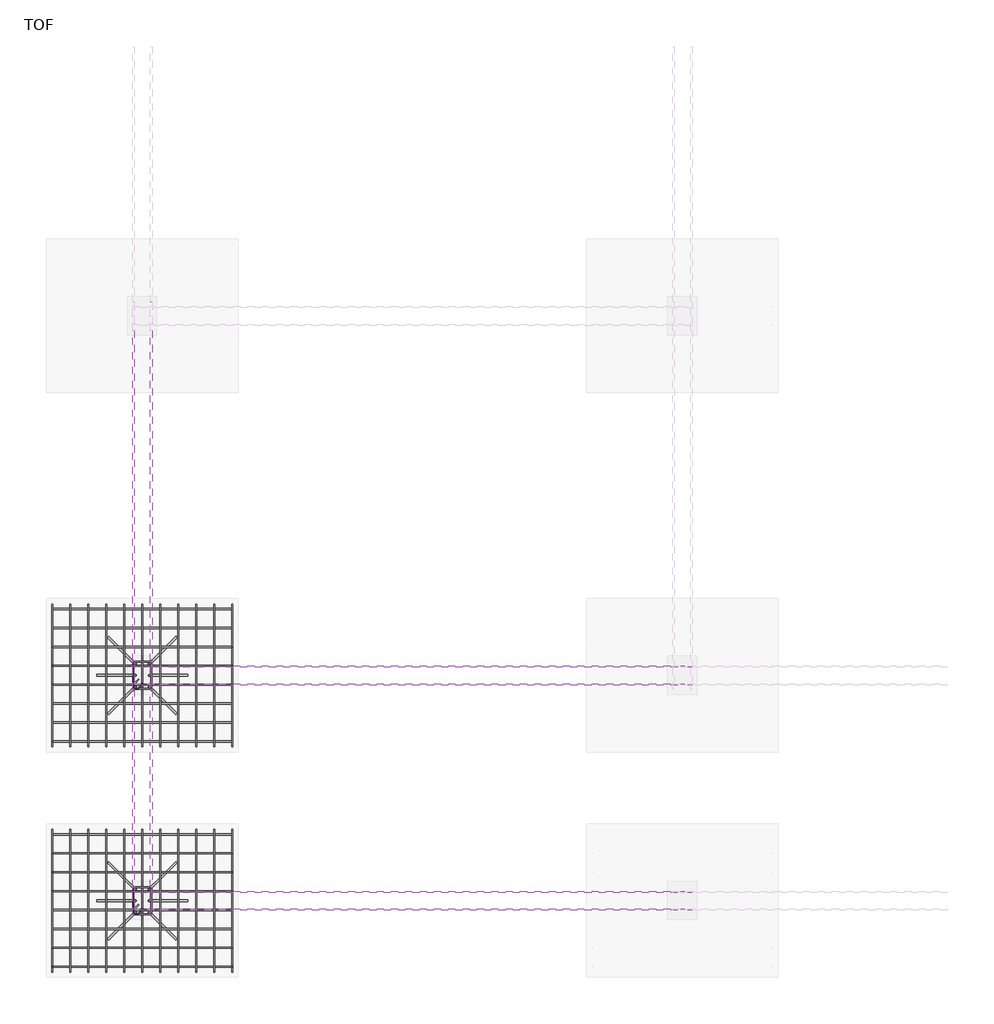
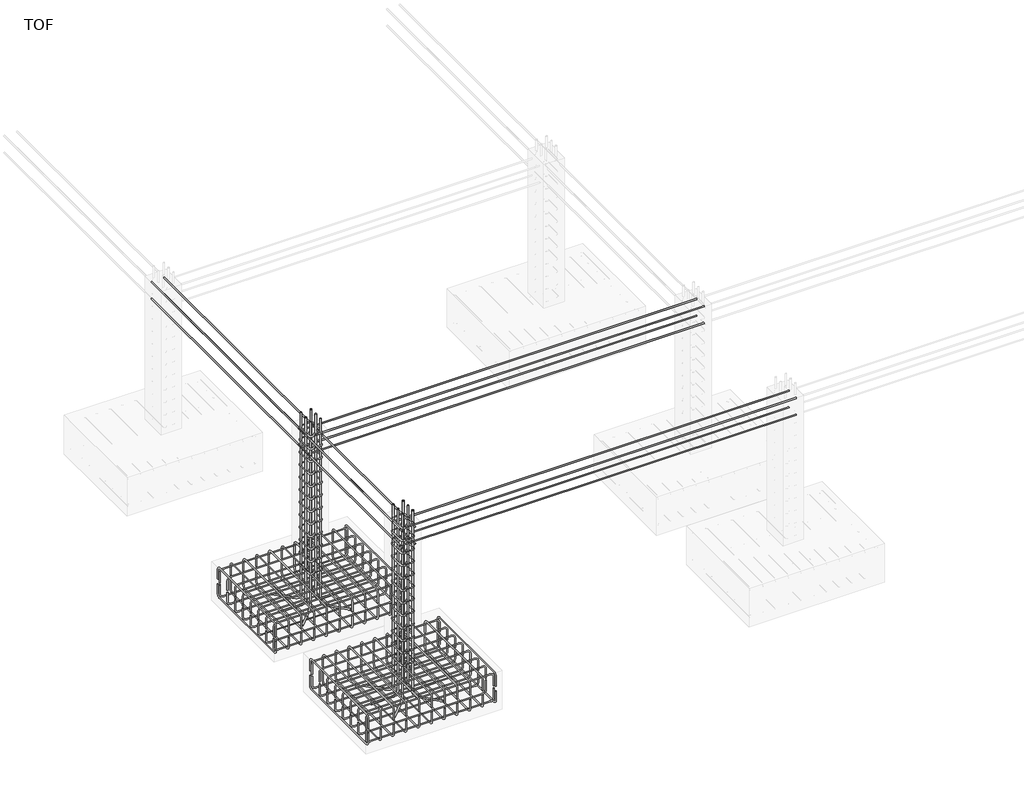
# One storey, part 2 of 10: 38 reinforcing bars.
"""IFC4 building model written with IfcOpenShell, lengths in millimetres."""

from ifc_helpers import new_model, si_unit, point, frame, origin, place, context, project, spatial, polyline, circle_curve, trimmed, segment, composite_curve, source, transform, mapped, element, save
from ifc_brep_helpers import swept_disk

model = new_model("IFC4")

# Units and contexts
model_context = context("Model", 3, world=origin())
ifc_project = project(units=[si_unit("LENGTHUNIT", "METRE", prefix="MILLI")], contexts=[model_context])

# Site, building, storey
site = spatial("IfcSite", under=ifc_project)
building = spatial("IfcBuilding", under=site)
storey = spatial("IfcBuildingStorey", under=building, Name="TOF", Elevation=-1828.8)

# Reinforcing bars
placement = place(None, origin())
reinforcing_bar_shape = source(origin(), model_context, "Body", "SolidModel", [
    swept_disk(composite_curve([segment(polyline([(-1914.7217857, -14539.6267376, -2018.8), (-1914.7217857, -14539.6267376, -1908.8)]), True, "CONTINUOUS"), segment(trimmed(circle_curve(frame((-1914.7217857, -14574.6267376, -1908.8), z_axis=(1.0, 0.0, 0.0), x_axis=(0.0, 35.0, 0.0)), 35.0), [point((-1914.7217857, -14539.6267376, -1908.8))], [point((-1914.7217857, -14574.6267376, -1873.8))], True, "CARTESIAN"), True, "CONTINUOUS"), segment(polyline([(-1914.7217857, -14574.6267376, -1873.8), (-1914.7217857, -15614.6267376, -1873.8)]), True, "CONTINUOUS"), segment(trimmed(circle_curve(frame((-1914.7217857, -15614.6267376, -1908.8), z_axis=(1.0, 0.0, 0.0), x_axis=(0.0, 0.0, 35.0)), 35.0), [point((-1914.7217857, -15614.6267376, -1873.8))], [point((-1914.7217857, -15649.6267376, -1908.8))], True, "CARTESIAN"), True, "CONTINUOUS"), segment(polyline([(-1914.7217857, -15649.6267376, -1908.8), (-1914.7217857, -15649.6267376, -2018.8)]), True, "CONTINUOUS")], self_intersect=False), 5.0),
])
element("IfcReinforcingBar", 1, at=placement, inside=storey, context=model_context, shape_type="MappedRepresentation", body=[
    mapped(reinforcing_bar_shape, transform((0.0, 0.0, 0.0), x_axis=(1.0, 0.0, 0.0), y_axis=(0.0, 1.0, 0.0), z_axis=(0.0, 0.0, 1.0))),
    mapped(reinforcing_bar_shape, transform((-141.0, 0.0, 0.0), x_axis=(1.0, 0.0, 0.0), y_axis=(0.0, 1.0, 0.0), z_axis=(0.0, 0.0, 1.0))),
    mapped(reinforcing_bar_shape, transform((-282.0, 0.0, 0.0), x_axis=(1.0, 0.0, 0.0), y_axis=(0.0, 1.0, 0.0), z_axis=(0.0, 0.0, 1.0))),
    mapped(reinforcing_bar_shape, transform((-423.0, 0.0, 0.0), x_axis=(1.0, 0.0, 0.0), y_axis=(0.0, 1.0, 0.0), z_axis=(0.0, 0.0, 1.0))),
    mapped(reinforcing_bar_shape, transform((-564.0, 0.0, 0.0), x_axis=(1.0, 0.0, 0.0), y_axis=(0.0, 1.0, 0.0), z_axis=(0.0, 0.0, 1.0))),
    mapped(reinforcing_bar_shape, transform((-705.0, 0.0, 0.0), x_axis=(1.0, 0.0, 0.0), y_axis=(0.0, 1.0, 0.0), z_axis=(0.0, 0.0, 1.0))),
    mapped(reinforcing_bar_shape, transform((-846.0, 0.0, 0.0), x_axis=(1.0, 0.0, 0.0), y_axis=(0.0, 1.0, 0.0), z_axis=(0.0, 0.0, 1.0))),
    mapped(reinforcing_bar_shape, transform((-987.0, 0.0, 0.0), x_axis=(1.0, 0.0, 0.0), y_axis=(0.0, 1.0, 0.0), z_axis=(0.0, 0.0, 1.0))),
    mapped(reinforcing_bar_shape, transform((-1128.0, 0.0, 0.0), x_axis=(1.0, 0.0, 0.0), y_axis=(0.0, 1.0, 0.0), z_axis=(0.0, 0.0, 1.0))),
    mapped(reinforcing_bar_shape, transform((-1269.0, 0.0, 0.0), x_axis=(1.0, 0.0, 0.0), y_axis=(0.0, 1.0, 0.0), z_axis=(0.0, 0.0, 1.0))),
    mapped(reinforcing_bar_shape, transform((-1410.0, 0.0, 0.0), x_axis=(1.0, 0.0, 0.0), y_axis=(0.0, 1.0, 0.0), z_axis=(0.0, 0.0, 1.0))),
])
reinforcing_bar_2_shape = source(origin(), model_context, "Body", "SolidModel", [
    swept_disk(composite_curve([segment(polyline([(-1914.7217857, -15649.6267376, -2077.5233378), (-1914.7217857, -15649.6267376, -2187.5233378)]), True, "CONTINUOUS"), segment(trimmed(circle_curve(frame((-1914.7217857, -15614.6267376, -2187.5233378), z_axis=(1.0, 0.0, 0.0), x_axis=(0.0, -35.0, 0.0)), 35.0), [point((-1914.7217857, -15649.6267376, -2187.5233378))], [point((-1914.7217857, -15614.6267376, -2222.5233378))], True, "CARTESIAN"), True, "CONTINUOUS"), segment(polyline([(-1914.7217857, -15614.6267376, -2222.5233378), (-1914.7217857, -14574.6267376, -2222.5233378)]), True, "CONTINUOUS"), segment(trimmed(circle_curve(frame((-1914.7217857, -14574.6267376, -2187.5233378), z_axis=(1.0, 0.0, 0.0), x_axis=(0.0, 0.0, -35.0)), 35.0), [point((-1914.7217857, -14574.6267376, -2222.5233378))], [point((-1914.7217857, -14539.6267376, -2187.5233378))], True, "CARTESIAN"), True, "CONTINUOUS"), segment(polyline([(-1914.7217857, -14539.6267376, -2187.5233378), (-1914.7217857, -14539.6267376, -2077.5233378)]), True, "CONTINUOUS")], self_intersect=False), 5.0),
])
element("IfcReinforcingBar", 2, at=placement, inside=storey, context=model_context, shape_type="MappedRepresentation", body=[
    mapped(reinforcing_bar_2_shape, transform((0.0, 0.0, 0.0), x_axis=(1.0, 0.0, 0.0), y_axis=(0.0, 1.0, 0.0), z_axis=(0.0, 0.0, 1.0))),
    mapped(reinforcing_bar_2_shape, transform((-141.0, 0.0, 0.0), x_axis=(1.0, 0.0, 0.0), y_axis=(0.0, 1.0, 0.0), z_axis=(0.0, 0.0, 1.0))),
    mapped(reinforcing_bar_2_shape, transform((-282.0, 0.0, 0.0), x_axis=(1.0, 0.0, 0.0), y_axis=(0.0, 1.0, 0.0), z_axis=(0.0, 0.0, 1.0))),
    mapped(reinforcing_bar_2_shape, transform((-423.0, 0.0, 0.0), x_axis=(1.0, 0.0, 0.0), y_axis=(0.0, 1.0, 0.0), z_axis=(0.0, 0.0, 1.0))),
    mapped(reinforcing_bar_2_shape, transform((-564.0, 0.0, 0.0), x_axis=(1.0, 0.0, 0.0), y_axis=(0.0, 1.0, 0.0), z_axis=(0.0, 0.0, 1.0))),
    mapped(reinforcing_bar_2_shape, transform((-705.0, 0.0, 0.0), x_axis=(1.0, 0.0, 0.0), y_axis=(0.0, 1.0, 0.0), z_axis=(0.0, 0.0, 1.0))),
    mapped(reinforcing_bar_2_shape, transform((-846.0, 0.0, 0.0), x_axis=(1.0, 0.0, 0.0), y_axis=(0.0, 1.0, 0.0), z_axis=(0.0, 0.0, 1.0))),
    mapped(reinforcing_bar_2_shape, transform((-987.0, 0.0, 0.0), x_axis=(1.0, 0.0, 0.0), y_axis=(0.0, 1.0, 0.0), z_axis=(0.0, 0.0, 1.0))),
    mapped(reinforcing_bar_2_shape, transform((-1128.0, 0.0, 0.0), x_axis=(1.0, 0.0, 0.0), y_axis=(0.0, 1.0, 0.0), z_axis=(0.0, 0.0, 1.0))),
    mapped(reinforcing_bar_2_shape, transform((-1269.0, 0.0, 0.0), x_axis=(1.0, 0.0, 0.0), y_axis=(0.0, 1.0, 0.0), z_axis=(0.0, 0.0, 1.0))),
    mapped(reinforcing_bar_2_shape, transform((-1410.0, 0.0, 0.0), x_axis=(1.0, 0.0, 0.0), y_axis=(0.0, 1.0, 0.0), z_axis=(0.0, 0.0, 1.0))),
])
reinforcing_bar_3_shape = source(origin(), model_context, "Body", "SolidModel", [
    swept_disk(composite_curve([segment(polyline([(-1914.7217857, -14574.6861459, -2066.1776706), (-1914.7217857, -14574.6861459, -2176.1776706)]), True, "CONTINUOUS"), segment(trimmed(circle_curve(frame((-1949.7217857, -14574.6861459, -2176.1776706), z_axis=(0.0, 1.0, 0.0), x_axis=(35.0, 0.0, 0.0)), 35.0), [point((-1914.7217857, -14574.6861459, -2176.1776706))], [point((-1949.7217857, -14574.6861459, -2211.1776706))], True, "CARTESIAN"), True, "CONTINUOUS"), segment(polyline([(-1949.7217857, -14574.6861459, -2211.1776706), (-3289.7217857, -14574.6861459, -2211.1776706)]), True, "CONTINUOUS"), segment(trimmed(circle_curve(frame((-3289.7217857, -14574.6861459, -2176.1776706), z_axis=(0.0, 1.0, 0.0), x_axis=(0.0, 0.0, -35.0)), 35.0), [point((-3289.7217857, -14574.6861459, -2211.1776706))], [point((-3324.7217857, -14574.6861459, -2176.1776706))], True, "CARTESIAN"), True, "CONTINUOUS"), segment(polyline([(-3324.7217857, -14574.6861459, -2176.1776706), (-3324.7217857, -14574.6861459, -2066.1776706)]), True, "CONTINUOUS")], self_intersect=False), 5.0),
])
element("IfcReinforcingBar", 3, at=placement, inside=storey, context=model_context, shape_type="MappedRepresentation", body=[
    mapped(reinforcing_bar_3_shape, transform((0.0, 0.0, 0.0), x_axis=(1.0, 0.0, 0.0), y_axis=(0.0, 1.0, 0.0), z_axis=(0.0, 0.0, 1.0))),
    mapped(reinforcing_bar_3_shape, transform((0.0, -148.0321606, 0.0), x_axis=(1.0, 0.0, 0.0), y_axis=(0.0, 1.0, 0.0), z_axis=(0.0, 0.0, 1.0))),
    mapped(reinforcing_bar_3_shape, transform((0.0, -296.0643211, 0.0), x_axis=(1.0, 0.0, 0.0), y_axis=(0.0, 1.0, 0.0), z_axis=(0.0, 0.0, 1.0))),
    mapped(reinforcing_bar_3_shape, transform((0.0, -444.0964817, 0.0), x_axis=(1.0, 0.0, 0.0), y_axis=(0.0, 1.0, 0.0), z_axis=(0.0, 0.0, 1.0))),
    mapped(reinforcing_bar_3_shape, transform((0.0, -592.1286423, 0.0), x_axis=(1.0, 0.0, 0.0), y_axis=(0.0, 1.0, 0.0), z_axis=(0.0, 0.0, 1.0))),
    mapped(reinforcing_bar_3_shape, transform((0.0, -740.1608029, 0.0), x_axis=(1.0, 0.0, 0.0), y_axis=(0.0, 1.0, 0.0), z_axis=(0.0, 0.0, 1.0))),
    mapped(reinforcing_bar_3_shape, transform((0.0, -888.1929634, 0.0), x_axis=(1.0, 0.0, 0.0), y_axis=(0.0, 1.0, 0.0), z_axis=(0.0, 0.0, 1.0))),
    mapped(reinforcing_bar_3_shape, transform((0.0, -1036.225124, 0.0), x_axis=(1.0, 0.0, 0.0), y_axis=(0.0, 1.0, 0.0), z_axis=(0.0, 0.0, 1.0))),
])
reinforcing_bar_4_shape = source(origin(), model_context, "Body", "SolidModel", [
    swept_disk(composite_curve([segment(polyline([(-1914.7217857, -15610.9112699, -2039.256778), (-1914.7217857, -15610.9112699, -1929.256778)]), True, "CONTINUOUS"), segment(trimmed(circle_curve(frame((-1949.7217857, -15610.9112699, -1929.256778), z_axis=(0.0, -1.0, 0.0), x_axis=(35.0, 0.0, 0.0)), 35.0), [point((-1914.7217857, -15610.9112699, -1929.256778))], [point((-1949.7217857, -15610.9112699, -1894.256778))], True, "CARTESIAN"), True, "CONTINUOUS"), segment(polyline([(-1949.7217857, -15610.9112699, -1894.256778), (-3289.7217857, -15610.9112699, -1894.256778)]), True, "CONTINUOUS"), segment(trimmed(circle_curve(frame((-3289.7217857, -15610.9112699, -1929.256778), z_axis=(0.0, -1.0, 0.0), x_axis=(0.0, 0.0, 35.0)), 35.0), [point((-3289.7217857, -15610.9112699, -1894.256778))], [point((-3324.7217857, -15610.9112699, -1929.256778))], True, "CARTESIAN"), True, "CONTINUOUS"), segment(polyline([(-3324.7217857, -15610.9112699, -1929.256778), (-3324.7217857, -15610.9112699, -2039.256778)]), True, "CONTINUOUS")], self_intersect=False), 5.0),
])
element("IfcReinforcingBar", 4, at=placement, inside=storey, context=model_context, shape_type="MappedRepresentation", body=[
    mapped(reinforcing_bar_4_shape, transform((0.0, 0.0, 0.0), x_axis=(1.0, 0.0, 0.0), y_axis=(0.0, 1.0, 0.0), z_axis=(0.0, 0.0, 1.0))),
    mapped(reinforcing_bar_4_shape, transform((0.0, 148.0321606, 0.0), x_axis=(1.0, 0.0, 0.0), y_axis=(0.0, 1.0, 0.0), z_axis=(0.0, 0.0, 1.0))),
    mapped(reinforcing_bar_4_shape, transform((0.0, 296.0643211, 0.0), x_axis=(1.0, 0.0, 0.0), y_axis=(0.0, 1.0, 0.0), z_axis=(0.0, 0.0, 1.0))),
    mapped(reinforcing_bar_4_shape, transform((0.0, 444.0964817, 0.0), x_axis=(1.0, 0.0, 0.0), y_axis=(0.0, 1.0, 0.0), z_axis=(0.0, 0.0, 1.0))),
    mapped(reinforcing_bar_4_shape, transform((0.0, 592.1286423, 0.0), x_axis=(1.0, 0.0, 0.0), y_axis=(0.0, 1.0, 0.0), z_axis=(0.0, 0.0, 1.0))),
    mapped(reinforcing_bar_4_shape, transform((0.0, 740.1608029, 0.0), x_axis=(1.0, 0.0, 0.0), y_axis=(0.0, 1.0, 0.0), z_axis=(0.0, 0.0, 1.0))),
    mapped(reinforcing_bar_4_shape, transform((0.0, 888.1929634, 0.0), x_axis=(1.0, 0.0, 0.0), y_axis=(0.0, 1.0, 0.0), z_axis=(0.0, 0.0, 1.0))),
    mapped(reinforcing_bar_4_shape, transform((0.0, 1036.225124, 0.0), x_axis=(1.0, 0.0, 0.0), y_axis=(0.0, 1.0, 0.0), z_axis=(0.0, 0.0, 1.0))),
])
reinforcing_bar_5_shape = source(origin(), model_context, "Body", "SolidModel", [
    swept_disk(composite_curve([segment(polyline([(-1914.7217857, -12774.6267376, -2018.8), (-1914.7217857, -12774.6267376, -1908.8)]), True, "CONTINUOUS"), segment(trimmed(circle_curve(frame((-1914.7217857, -12809.6267376, -1908.8), z_axis=(1.0, 0.0, 0.0), x_axis=(0.0, 35.0, 0.0)), 35.0), [point((-1914.7217857, -12774.6267376, -1908.8))], [point((-1914.7217857, -12809.6267376, -1873.8))], True, "CARTESIAN"), True, "CONTINUOUS"), segment(polyline([(-1914.7217857, -12809.6267376, -1873.8), (-1914.7217857, -13849.6267376, -1873.8)]), True, "CONTINUOUS"), segment(trimmed(circle_curve(frame((-1914.7217857, -13849.6267376, -1908.8), z_axis=(1.0, 0.0, 0.0), x_axis=(0.0, 0.0, 35.0)), 35.0), [point((-1914.7217857, -13849.6267376, -1873.8))], [point((-1914.7217857, -13884.6267376, -1908.8))], True, "CARTESIAN"), True, "CONTINUOUS"), segment(polyline([(-1914.7217857, -13884.6267376, -1908.8), (-1914.7217857, -13884.6267376, -2018.8)]), True, "CONTINUOUS")], self_intersect=False), 5.0),
])
element("IfcReinforcingBar", 5, at=placement, inside=storey, context=model_context, shape_type="MappedRepresentation", body=[
    mapped(reinforcing_bar_5_shape, transform((0.0, 0.0, 0.0), x_axis=(1.0, 0.0, 0.0), y_axis=(0.0, 1.0, 0.0), z_axis=(0.0, 0.0, 1.0))),
    mapped(reinforcing_bar_5_shape, transform((-141.0, 0.0, 0.0), x_axis=(1.0, 0.0, 0.0), y_axis=(0.0, 1.0, 0.0), z_axis=(0.0, 0.0, 1.0))),
    mapped(reinforcing_bar_5_shape, transform((-282.0, 0.0, 0.0), x_axis=(1.0, 0.0, 0.0), y_axis=(0.0, 1.0, 0.0), z_axis=(0.0, 0.0, 1.0))),
    mapped(reinforcing_bar_5_shape, transform((-423.0, 0.0, 0.0), x_axis=(1.0, 0.0, 0.0), y_axis=(0.0, 1.0, 0.0), z_axis=(0.0, 0.0, 1.0))),
    mapped(reinforcing_bar_5_shape, transform((-564.0, 0.0, 0.0), x_axis=(1.0, 0.0, 0.0), y_axis=(0.0, 1.0, 0.0), z_axis=(0.0, 0.0, 1.0))),
    mapped(reinforcing_bar_5_shape, transform((-705.0, 0.0, 0.0), x_axis=(1.0, 0.0, 0.0), y_axis=(0.0, 1.0, 0.0), z_axis=(0.0, 0.0, 1.0))),
    mapped(reinforcing_bar_5_shape, transform((-846.0, 0.0, 0.0), x_axis=(1.0, 0.0, 0.0), y_axis=(0.0, 1.0, 0.0), z_axis=(0.0, 0.0, 1.0))),
    mapped(reinforcing_bar_5_shape, transform((-987.0, 0.0, 0.0), x_axis=(1.0, 0.0, 0.0), y_axis=(0.0, 1.0, 0.0), z_axis=(0.0, 0.0, 1.0))),
    mapped(reinforcing_bar_5_shape, transform((-1128.0, 0.0, 0.0), x_axis=(1.0, 0.0, 0.0), y_axis=(0.0, 1.0, 0.0), z_axis=(0.0, 0.0, 1.0))),
    mapped(reinforcing_bar_5_shape, transform((-1269.0, 0.0, 0.0), x_axis=(1.0, 0.0, 0.0), y_axis=(0.0, 1.0, 0.0), z_axis=(0.0, 0.0, 1.0))),
    mapped(reinforcing_bar_5_shape, transform((-1410.0, 0.0, 0.0), x_axis=(1.0, 0.0, 0.0), y_axis=(0.0, 1.0, 0.0), z_axis=(0.0, 0.0, 1.0))),
])
reinforcing_bar_6_shape = source(origin(), model_context, "Body", "SolidModel", [
    swept_disk(composite_curve([segment(polyline([(-1914.7217857, -13884.6267376, -2077.5233378), (-1914.7217857, -13884.6267376, -2187.5233378)]), True, "CONTINUOUS"), segment(trimmed(circle_curve(frame((-1914.7217857, -13849.6267376, -2187.5233378), z_axis=(1.0, 0.0, 0.0), x_axis=(0.0, -35.0, 0.0)), 35.0), [point((-1914.7217857, -13884.6267376, -2187.5233378))], [point((-1914.7217857, -13849.6267376, -2222.5233378))], True, "CARTESIAN"), True, "CONTINUOUS"), segment(polyline([(-1914.7217857, -13849.6267376, -2222.5233378), (-1914.7217857, -12809.6267376, -2222.5233378)]), True, "CONTINUOUS"), segment(trimmed(circle_curve(frame((-1914.7217857, -12809.6267376, -2187.5233378), z_axis=(1.0, 0.0, 0.0), x_axis=(0.0, 0.0, -35.0)), 35.0), [point((-1914.7217857, -12809.6267376, -2222.5233378))], [point((-1914.7217857, -12774.6267376, -2187.5233378))], True, "CARTESIAN"), True, "CONTINUOUS"), segment(polyline([(-1914.7217857, -12774.6267376, -2187.5233378), (-1914.7217857, -12774.6267376, -2077.5233378)]), True, "CONTINUOUS")], self_intersect=False), 5.0),
])
element("IfcReinforcingBar", 6, at=placement, inside=storey, context=model_context, shape_type="MappedRepresentation", body=[
    mapped(reinforcing_bar_6_shape, transform((0.0, 0.0, 0.0), x_axis=(1.0, 0.0, 0.0), y_axis=(0.0, 1.0, 0.0), z_axis=(0.0, 0.0, 1.0))),
    mapped(reinforcing_bar_6_shape, transform((-141.0, 0.0, 0.0), x_axis=(1.0, 0.0, 0.0), y_axis=(0.0, 1.0, 0.0), z_axis=(0.0, 0.0, 1.0))),
    mapped(reinforcing_bar_6_shape, transform((-282.0, 0.0, 0.0), x_axis=(1.0, 0.0, 0.0), y_axis=(0.0, 1.0, 0.0), z_axis=(0.0, 0.0, 1.0))),
    mapped(reinforcing_bar_6_shape, transform((-423.0, 0.0, 0.0), x_axis=(1.0, 0.0, 0.0), y_axis=(0.0, 1.0, 0.0), z_axis=(0.0, 0.0, 1.0))),
    mapped(reinforcing_bar_6_shape, transform((-564.0, 0.0, 0.0), x_axis=(1.0, 0.0, 0.0), y_axis=(0.0, 1.0, 0.0), z_axis=(0.0, 0.0, 1.0))),
    mapped(reinforcing_bar_6_shape, transform((-705.0, 0.0, 0.0), x_axis=(1.0, 0.0, 0.0), y_axis=(0.0, 1.0, 0.0), z_axis=(0.0, 0.0, 1.0))),
    mapped(reinforcing_bar_6_shape, transform((-846.0, 0.0, 0.0), x_axis=(1.0, 0.0, 0.0), y_axis=(0.0, 1.0, 0.0), z_axis=(0.0, 0.0, 1.0))),
    mapped(reinforcing_bar_6_shape, transform((-987.0, 0.0, 0.0), x_axis=(1.0, 0.0, 0.0), y_axis=(0.0, 1.0, 0.0), z_axis=(0.0, 0.0, 1.0))),
    mapped(reinforcing_bar_6_shape, transform((-1128.0, 0.0, 0.0), x_axis=(1.0, 0.0, 0.0), y_axis=(0.0, 1.0, 0.0), z_axis=(0.0, 0.0, 1.0))),
    mapped(reinforcing_bar_6_shape, transform((-1269.0, 0.0, 0.0), x_axis=(1.0, 0.0, 0.0), y_axis=(0.0, 1.0, 0.0), z_axis=(0.0, 0.0, 1.0))),
    mapped(reinforcing_bar_6_shape, transform((-1410.0, 0.0, 0.0), x_axis=(1.0, 0.0, 0.0), y_axis=(0.0, 1.0, 0.0), z_axis=(0.0, 0.0, 1.0))),
])
reinforcing_bar_7_shape = source(origin(), model_context, "Body", "SolidModel", [
    swept_disk(composite_curve([segment(polyline([(-1914.7217857, -12809.6861459, -2066.1776706), (-1914.7217857, -12809.6861459, -2176.1776706)]), True, "CONTINUOUS"), segment(trimmed(circle_curve(frame((-1949.7217857, -12809.6861459, -2176.1776706), z_axis=(0.0, 1.0, 0.0), x_axis=(35.0, 0.0, 0.0)), 35.0), [point((-1914.7217857, -12809.6861459, -2176.1776706))], [point((-1949.7217857, -12809.6861459, -2211.1776706))], True, "CARTESIAN"), True, "CONTINUOUS"), segment(polyline([(-1949.7217857, -12809.6861459, -2211.1776706), (-3289.7217857, -12809.6861459, -2211.1776706)]), True, "CONTINUOUS"), segment(trimmed(circle_curve(frame((-3289.7217857, -12809.6861459, -2176.1776706), z_axis=(0.0, 1.0, 0.0), x_axis=(0.0, 0.0, -35.0)), 35.0), [point((-3289.7217857, -12809.6861459, -2211.1776706))], [point((-3324.7217857, -12809.6861459, -2176.1776706))], True, "CARTESIAN"), True, "CONTINUOUS"), segment(polyline([(-3324.7217857, -12809.6861459, -2176.1776706), (-3324.7217857, -12809.6861459, -2066.1776706)]), True, "CONTINUOUS")], self_intersect=False), 5.0),
])
element("IfcReinforcingBar", 7, at=placement, inside=storey, context=model_context, shape_type="MappedRepresentation", body=[
    mapped(reinforcing_bar_7_shape, transform((0.0, 0.0, 0.0), x_axis=(1.0, 0.0, 0.0), y_axis=(0.0, 1.0, 0.0), z_axis=(0.0, 0.0, 1.0))),
    mapped(reinforcing_bar_7_shape, transform((0.0, -148.0321606, 0.0), x_axis=(1.0, 0.0, 0.0), y_axis=(0.0, 1.0, 0.0), z_axis=(0.0, 0.0, 1.0))),
    mapped(reinforcing_bar_7_shape, transform((0.0, -296.0643211, 0.0), x_axis=(1.0, 0.0, 0.0), y_axis=(0.0, 1.0, 0.0), z_axis=(0.0, 0.0, 1.0))),
    mapped(reinforcing_bar_7_shape, transform((0.0, -444.0964817, 0.0), x_axis=(1.0, 0.0, 0.0), y_axis=(0.0, 1.0, 0.0), z_axis=(0.0, 0.0, 1.0))),
    mapped(reinforcing_bar_7_shape, transform((0.0, -592.1286423, 0.0), x_axis=(1.0, 0.0, 0.0), y_axis=(0.0, 1.0, 0.0), z_axis=(0.0, 0.0, 1.0))),
    mapped(reinforcing_bar_7_shape, transform((0.0, -740.1608029, 0.0), x_axis=(1.0, 0.0, 0.0), y_axis=(0.0, 1.0, 0.0), z_axis=(0.0, 0.0, 1.0))),
    mapped(reinforcing_bar_7_shape, transform((0.0, -888.1929634, 0.0), x_axis=(1.0, 0.0, 0.0), y_axis=(0.0, 1.0, 0.0), z_axis=(0.0, 0.0, 1.0))),
    mapped(reinforcing_bar_7_shape, transform((0.0, -1036.225124, 0.0), x_axis=(1.0, 0.0, 0.0), y_axis=(0.0, 1.0, 0.0), z_axis=(0.0, 0.0, 1.0))),
])
reinforcing_bar_8_shape = source(origin(), model_context, "Body", "SolidModel", [
    swept_disk(composite_curve([segment(polyline([(-1914.7217857, -13845.9112699, -2039.256778), (-1914.7217857, -13845.9112699, -1929.256778)]), True, "CONTINUOUS"), segment(trimmed(circle_curve(frame((-1949.7217857, -13845.9112699, -1929.256778), z_axis=(0.0, -1.0, 0.0), x_axis=(35.0, 0.0, 0.0)), 35.0), [point((-1914.7217857, -13845.9112699, -1929.256778))], [point((-1949.7217857, -13845.9112699, -1894.256778))], True, "CARTESIAN"), True, "CONTINUOUS"), segment(polyline([(-1949.7217857, -13845.9112699, -1894.256778), (-3289.7217857, -13845.9112699, -1894.256778)]), True, "CONTINUOUS"), segment(trimmed(circle_curve(frame((-3289.7217857, -13845.9112699, -1929.256778), z_axis=(0.0, -1.0, 0.0), x_axis=(0.0, 0.0, 35.0)), 35.0), [point((-3289.7217857, -13845.9112699, -1894.256778))], [point((-3324.7217857, -13845.9112699, -1929.256778))], True, "CARTESIAN"), True, "CONTINUOUS"), segment(polyline([(-3324.7217857, -13845.9112699, -1929.256778), (-3324.7217857, -13845.9112699, -2039.256778)]), True, "CONTINUOUS")], self_intersect=False), 5.0),
])
element("IfcReinforcingBar", 8, at=placement, inside=storey, context=model_context, shape_type="MappedRepresentation", body=[
    mapped(reinforcing_bar_8_shape, transform((0.0, 0.0, 0.0), x_axis=(1.0, 0.0, 0.0), y_axis=(0.0, 1.0, 0.0), z_axis=(0.0, 0.0, 1.0))),
    mapped(reinforcing_bar_8_shape, transform((0.0, 148.0321606, 0.0), x_axis=(1.0, 0.0, 0.0), y_axis=(0.0, 1.0, 0.0), z_axis=(0.0, 0.0, 1.0))),
    mapped(reinforcing_bar_8_shape, transform((0.0, 296.0643211, 0.0), x_axis=(1.0, 0.0, 0.0), y_axis=(0.0, 1.0, 0.0), z_axis=(0.0, 0.0, 1.0))),
    mapped(reinforcing_bar_8_shape, transform((0.0, 444.0964817, 0.0), x_axis=(1.0, 0.0, 0.0), y_axis=(0.0, 1.0, 0.0), z_axis=(0.0, 0.0, 1.0))),
    mapped(reinforcing_bar_8_shape, transform((0.0, 592.1286423, 0.0), x_axis=(1.0, 0.0, 0.0), y_axis=(0.0, 1.0, 0.0), z_axis=(0.0, 0.0, 1.0))),
    mapped(reinforcing_bar_8_shape, transform((0.0, 740.1608029, 0.0), x_axis=(1.0, 0.0, 0.0), y_axis=(0.0, 1.0, 0.0), z_axis=(0.0, 0.0, 1.0))),
    mapped(reinforcing_bar_8_shape, transform((0.0, 888.1929634, 0.0), x_axis=(1.0, 0.0, 0.0), y_axis=(0.0, 1.0, 0.0), z_axis=(0.0, 0.0, 1.0))),
    mapped(reinforcing_bar_8_shape, transform((0.0, 1036.225124, 0.0), x_axis=(1.0, 0.0, 0.0), y_axis=(0.0, 1.0, 0.0), z_axis=(0.0, 0.0, 1.0))),
])
reinforcing_bar_9_shape = source(origin(), model_context, "Body", "SolidModel", [
    swept_disk(composite_curve([segment(polyline([(-2649.751223, -15125.7150493, -1784.8), (-2683.6923485, -15159.6561748, -1784.8)]), True, "CONTINUOUS"), segment(trimmed(circle_curve(frame((-2666.7217857, -15176.6267376, -1784.8), z_axis=(0.0, 0.0, 1.0), x_axis=(-16.970562800000152, 16.970562799999243, 0.0)), 24.0), [point((-2683.6923485, -15159.6561748, -1784.8))], [point((-2666.7217857, -15200.6267376, -1784.8))], True, "CARTESIAN"), True, "CONTINUOUS"), segment(polyline([(-2666.7217857, -15200.6267376, -1784.8), (-2572.7217857, -15200.6267376, -1784.8)]), True, "CONTINUOUS"), segment(trimmed(circle_curve(frame((-2572.7217857, -15176.6267376, -1784.8), z_axis=(0.0, 0.0, 1.0), x_axis=(0.0, -24.0, 0.0)), 24.0), [point((-2572.7217857, -15200.6267376, -1784.8))], [point((-2548.7217857, -15176.6267376, -1784.8))], True, "CARTESIAN"), True, "CONTINUOUS"), segment(polyline([(-2548.7217857, -15176.6267376, -1784.8), (-2548.7217857, -15012.6267376, -1784.8)]), True, "CONTINUOUS"), segment(trimmed(circle_curve(frame((-2572.6837885, -15012.6267376, -1786.149972), z_axis=(-0.05624883273897078, 0.0, 0.9984167811167355), x_axis=(23.962002799999937, 0.0, 1.3499719999999797)), 24.0), [point((-2548.7217857, -15012.6267376, -1784.8))], [point((-2572.6837885, -14988.6267376, -1786.149972))], True, "CARTESIAN"), True, "CONTINUOUS"), segment(polyline([(-2572.6837885, -14988.6267376, -1786.149972), (-2666.759783, -14988.6267376, -1791.450028)]), True, "CONTINUOUS"), segment(trimmed(circle_curve(frame((-2666.759783, -15012.6267376, -1791.450028), z_axis=(-0.05624883273897078, 0.0, 0.9984167811167355), x_axis=(0.0, 24.0, 0.0)), 24.0), [point((-2666.759783, -14988.6267376, -1791.450028))], [point((-2690.7217857, -15012.6267376, -1792.8))], True, "CARTESIAN"), True, "CONTINUOUS"), segment(polyline([(-2690.7217857, -15012.6267376, -1792.8), (-2690.7217857, -15176.6267376, -1792.8)]), True, "CONTINUOUS"), segment(trimmed(circle_curve(frame((-2666.7217857, -15176.6267376, -1792.8), z_axis=(0.0, 0.0, 1.0), x_axis=(-24.0, 0.0, 0.0)), 24.0), [point((-2690.7217857, -15176.6267376, -1792.8))], [point((-2649.751223, -15193.5973003, -1792.8))], True, "CARTESIAN"), True, "CONTINUOUS"), segment(polyline([(-2649.751223, -15193.5973003, -1792.8), (-2615.8100975, -15159.6561748, -1792.8)]), True, "CONTINUOUS")], self_intersect=False), 4.0),
])
element("IfcReinforcingBar", 9, at=placement, inside=storey, context=model_context, shape_type="MappedRepresentation", body=[
    mapped(reinforcing_bar_9_shape, transform((0.0, 0.0, 0.0), x_axis=(1.0, 0.0, 0.0), y_axis=(0.0, 1.0, 0.0), z_axis=(0.0, 0.0, 1.0))),
    mapped(reinforcing_bar_9_shape, transform((0.0, 0.0, 145.9395608), x_axis=(1.0, 0.0, 0.0), y_axis=(0.0, 1.0, 0.0), z_axis=(0.0, 0.0, 1.0))),
    mapped(reinforcing_bar_9_shape, transform((0.0, 0.0, 291.8791216), x_axis=(1.0, 0.0, 0.0), y_axis=(0.0, 1.0, 0.0), z_axis=(0.0, 0.0, 1.0))),
    mapped(reinforcing_bar_9_shape, transform((0.0, 0.0, 437.8186825), x_axis=(1.0, 0.0, 0.0), y_axis=(0.0, 1.0, 0.0), z_axis=(0.0, 0.0, 1.0))),
    mapped(reinforcing_bar_9_shape, transform((0.0, 0.0, 583.7582433), x_axis=(1.0, 0.0, 0.0), y_axis=(0.0, 1.0, 0.0), z_axis=(0.0, 0.0, 1.0))),
    mapped(reinforcing_bar_9_shape, transform((0.0, 0.0, 729.6978041), x_axis=(1.0, 0.0, 0.0), y_axis=(0.0, 1.0, 0.0), z_axis=(0.0, 0.0, 1.0))),
    mapped(reinforcing_bar_9_shape, transform((0.0, 0.0, 875.6373649), x_axis=(1.0, 0.0, 0.0), y_axis=(0.0, 1.0, 0.0), z_axis=(0.0, 0.0, 1.0))),
    mapped(reinforcing_bar_9_shape, transform((0.0, 0.0, 1021.5769258), x_axis=(1.0, 0.0, 0.0), y_axis=(0.0, 1.0, 0.0), z_axis=(0.0, 0.0, 1.0))),
    mapped(reinforcing_bar_9_shape, transform((0.0, 0.0, 1167.5164866), x_axis=(1.0, 0.0, 0.0), y_axis=(0.0, 1.0, 0.0), z_axis=(0.0, 0.0, 1.0))),
    mapped(reinforcing_bar_9_shape, transform((0.0, 0.0, 1313.4560474), x_axis=(1.0, 0.0, 0.0), y_axis=(0.0, 1.0, 0.0), z_axis=(0.0, 0.0, 1.0))),
    mapped(reinforcing_bar_9_shape, transform((0.0, 0.0, 1459.3956082), x_axis=(1.0, 0.0, 0.0), y_axis=(0.0, 1.0, 0.0), z_axis=(0.0, 0.0, 1.0))),
    mapped(reinforcing_bar_9_shape, transform((0.0, 0.0, 1605.3351691), x_axis=(1.0, 0.0, 0.0), y_axis=(0.0, 1.0, 0.0), z_axis=(0.0, 0.0, 1.0))),
])
element("IfcReinforcingBar", 10, at=placement, inside=storey, context=model_context, shape_type="SolidModel", body=[
    swept_disk(composite_curve([segment(polyline([(-2564.115184, -15185.2333393, -20.0), (-2564.115184, -15185.2333393, -2138.7824747)]), True, "CONTINUOUS"), segment(trimmed(circle_curve(frame((-2524.8707576, -15224.4777657, -2138.7824747), z_axis=(-0.7071067811865545, -0.7071067811865406, 0.0), x_axis=(-39.244426400000066, 39.2444263999987, 0.0)), 55.5), [point((-2564.115184, -15185.2333393, -2138.7824747))], [point((-2524.8707576, -15224.4777657, -2194.2824747))], True, "CARTESIAN"), True, "CONTINUOUS"), segment(polyline([(-2524.8707576, -15224.4777657, -2194.2824747), (-2352.4916085, -15396.8569148, -2194.2824747)]), True, "CONTINUOUS")], self_intersect=False), 8.0),
])
element("IfcReinforcingBar", 11, at=placement, inside=storey, context=model_context, shape_type="SolidModel", body=[
    swept_disk(composite_curve([segment(polyline([(-2564.065184, -15094.6267376, -20.0), (-2564.065184, -15094.6267376, -2138.7824747)]), True, "CONTINUOUS"), segment(trimmed(circle_curve(frame((-2508.565184, -15094.6267376, -2138.7824747), z_axis=(0.0, -1.0, 0.0), x_axis=(-55.5, 0.0, 0.0)), 55.5), [point((-2564.065184, -15094.6267376, -2138.7824747))], [point((-2508.565184, -15094.6267376, -2194.2824747))], True, "CARTESIAN"), True, "CONTINUOUS"), segment(polyline([(-2508.565184, -15094.6267376, -2194.2824747), (-2264.8342534, -15094.6267376, -2194.2824747)]), True, "CONTINUOUS")], self_intersect=False), 8.0),
])
element("IfcReinforcingBar", 12, at=placement, inside=storey, context=model_context, shape_type="SolidModel", body=[
    swept_disk(composite_curve([segment(polyline([(-2564.115184, -15004.0201359, -20.0), (-2564.115184, -15004.0201359, -2138.7824747)]), True, "CONTINUOUS"), segment(trimmed(circle_curve(frame((-2524.8707576, -14964.7757095, -2138.7824747), z_axis=(0.7071067811865545, -0.7071067811865407, 0.0), x_axis=(-39.244426400000066, -39.24442640000052, 0.0)), 55.5), [point((-2564.115184, -15004.0201359, -2138.7824747))], [point((-2524.8707576, -14964.7757095, -2194.2824747))], True, "CARTESIAN"), True, "CONTINUOUS"), segment(polyline([(-2524.8707576, -14964.7757095, -2194.2824747), (-2352.4916085, -14792.3965603, -2194.2824747)]), True, "CONTINUOUS")], self_intersect=False), 8.0),
])
element("IfcReinforcingBar", 13, at=placement, inside=storey, context=model_context, shape_type="SolidModel", body=[
    swept_disk(composite_curve([segment(polyline([(-2675.3283874, -15185.2333393, -20.0), (-2675.3283874, -15185.2333393, -2138.7824747)]), True, "CONTINUOUS"), segment(trimmed(circle_curve(frame((-2714.5728138, -15224.4777657, -2138.7824747), z_axis=(-0.7071067811865517, 0.7071067811865434, 0.0), x_axis=(39.244426400000066, 39.2444263999987, 0.0)), 55.5), [point((-2675.3283874, -15185.2333393, -2138.7824747))], [point((-2714.5728138, -15224.4777657, -2194.2824747))], True, "CARTESIAN"), True, "CONTINUOUS"), segment(polyline([(-2714.5728138, -15224.4777657, -2194.2824747), (-2886.951963, -15396.8569148, -2194.2824747)]), True, "CONTINUOUS")], self_intersect=False), 8.0),
])
element("IfcReinforcingBar", 14, at=placement, inside=storey, context=model_context, shape_type="SolidModel", body=[
    swept_disk(composite_curve([segment(polyline([(-2675.3783874, -15094.6267376, -20.0), (-2675.3783874, -15094.6267376, -2138.7824747)]), True, "CONTINUOUS"), segment(trimmed(circle_curve(frame((-2730.8783874, -15094.6267376, -2138.7824747), z_axis=(0.0, 1.0, 0.0), x_axis=(55.5, 0.0, 0.0)), 55.5), [point((-2675.3783874, -15094.6267376, -2138.7824747))], [point((-2730.8783874, -15094.6267376, -2194.2824747))], True, "CARTESIAN"), True, "CONTINUOUS"), segment(polyline([(-2730.8783874, -15094.6267376, -2194.2824747), (-2974.6093181, -15094.6267376, -2194.2824747)]), True, "CONTINUOUS")], self_intersect=False), 8.0),
])
element("IfcReinforcingBar", 15, at=placement, inside=storey, context=model_context, shape_type="SolidModel", body=[
    swept_disk(composite_curve([segment(polyline([(-2675.3283874, -15004.0201359, -20.0), (-2675.3283874, -15004.0201359, -2138.7824747)]), True, "CONTINUOUS"), segment(trimmed(circle_curve(frame((-2714.5728138, -14964.7757095, -2138.7824747), z_axis=(0.7071067811865572, 0.7071067811865379, 0.0), x_axis=(39.244426400000066, -39.24442640000052, 0.0)), 55.5), [point((-2675.3283874, -15004.0201359, -2138.7824747))], [point((-2714.5728138, -14964.7757095, -2194.2824747))], True, "CARTESIAN"), True, "CONTINUOUS"), segment(polyline([(-2714.5728138, -14964.7757095, -2194.2824747), (-2886.951963, -14792.3965603, -2194.2824747)]), True, "CONTINUOUS")], self_intersect=False), 8.0),
])
reinforcing_bar_10_shape = source(origin(), model_context, "Body", "SolidModel", [
    swept_disk(composite_curve([segment(polyline([(-2649.751223, -13360.7150493, -1784.8), (-2683.6923485, -13394.6561748, -1784.8)]), True, "CONTINUOUS"), segment(trimmed(circle_curve(frame((-2666.7217857, -13411.6267376, -1784.8), z_axis=(0.0, 0.0, 1.0), x_axis=(-16.970562800000152, 16.970562799999243, 0.0)), 24.0), [point((-2683.6923485, -13394.6561748, -1784.8))], [point((-2666.7217857, -13435.6267376, -1784.8))], True, "CARTESIAN"), True, "CONTINUOUS"), segment(polyline([(-2666.7217857, -13435.6267376, -1784.8), (-2572.7217857, -13435.6267376, -1784.8)]), True, "CONTINUOUS"), segment(trimmed(circle_curve(frame((-2572.7217857, -13411.6267376, -1784.8), z_axis=(0.0, 0.0, 1.0), x_axis=(0.0, -24.0, 0.0)), 24.0), [point((-2572.7217857, -13435.6267376, -1784.8))], [point((-2548.7217857, -13411.6267376, -1784.8))], True, "CARTESIAN"), True, "CONTINUOUS"), segment(polyline([(-2548.7217857, -13411.6267376, -1784.8), (-2548.7217857, -13247.6267376, -1784.8)]), True, "CONTINUOUS"), segment(trimmed(circle_curve(frame((-2572.6837885, -13247.6267376, -1786.149972), z_axis=(-0.05624883273897078, 0.0, 0.9984167811167355), x_axis=(23.962002799999937, 0.0, 1.3499719999999797)), 24.0), [point((-2548.7217857, -13247.6267376, -1784.8))], [point((-2572.6837885, -13223.6267376, -1786.149972))], True, "CARTESIAN"), True, "CONTINUOUS"), segment(polyline([(-2572.6837885, -13223.6267376, -1786.149972), (-2666.759783, -13223.6267376, -1791.450028)]), True, "CONTINUOUS"), segment(trimmed(circle_curve(frame((-2666.759783, -13247.6267376, -1791.450028), z_axis=(-0.05624883273897078, 0.0, 0.9984167811167355), x_axis=(0.0, 24.0, 0.0)), 24.0), [point((-2666.759783, -13223.6267376, -1791.450028))], [point((-2690.7217857, -13247.6267376, -1792.8))], True, "CARTESIAN"), True, "CONTINUOUS"), segment(polyline([(-2690.7217857, -13247.6267376, -1792.8), (-2690.7217857, -13411.6267376, -1792.8)]), True, "CONTINUOUS"), segment(trimmed(circle_curve(frame((-2666.7217857, -13411.6267376, -1792.8), z_axis=(0.0, 0.0, 1.0), x_axis=(-24.0, 0.0, 0.0)), 24.0), [point((-2690.7217857, -13411.6267376, -1792.8))], [point((-2649.751223, -13428.5973003, -1792.8))], True, "CARTESIAN"), True, "CONTINUOUS"), segment(polyline([(-2649.751223, -13428.5973003, -1792.8), (-2615.8100975, -13394.6561748, -1792.8)]), True, "CONTINUOUS")], self_intersect=False), 4.0),
])
element("IfcReinforcingBar", 16, at=placement, inside=storey, context=model_context, shape_type="MappedRepresentation", body=[
    mapped(reinforcing_bar_10_shape, transform((0.0, 0.0, 0.0), x_axis=(1.0, 0.0, 0.0), y_axis=(0.0, 1.0, 0.0), z_axis=(0.0, 0.0, 1.0))),
    mapped(reinforcing_bar_10_shape, transform((0.0, 0.0, 145.9395608), x_axis=(1.0, 0.0, 0.0), y_axis=(0.0, 1.0, 0.0), z_axis=(0.0, 0.0, 1.0))),
    mapped(reinforcing_bar_10_shape, transform((0.0, 0.0, 291.8791216), x_axis=(1.0, 0.0, 0.0), y_axis=(0.0, 1.0, 0.0), z_axis=(0.0, 0.0, 1.0))),
    mapped(reinforcing_bar_10_shape, transform((0.0, 0.0, 437.8186825), x_axis=(1.0, 0.0, 0.0), y_axis=(0.0, 1.0, 0.0), z_axis=(0.0, 0.0, 1.0))),
    mapped(reinforcing_bar_10_shape, transform((0.0, 0.0, 583.7582433), x_axis=(1.0, 0.0, 0.0), y_axis=(0.0, 1.0, 0.0), z_axis=(0.0, 0.0, 1.0))),
    mapped(reinforcing_bar_10_shape, transform((0.0, 0.0, 729.6978041), x_axis=(1.0, 0.0, 0.0), y_axis=(0.0, 1.0, 0.0), z_axis=(0.0, 0.0, 1.0))),
    mapped(reinforcing_bar_10_shape, transform((0.0, 0.0, 875.6373649), x_axis=(1.0, 0.0, 0.0), y_axis=(0.0, 1.0, 0.0), z_axis=(0.0, 0.0, 1.0))),
    mapped(reinforcing_bar_10_shape, transform((0.0, 0.0, 1021.5769258), x_axis=(1.0, 0.0, 0.0), y_axis=(0.0, 1.0, 0.0), z_axis=(0.0, 0.0, 1.0))),
    mapped(reinforcing_bar_10_shape, transform((0.0, 0.0, 1167.5164866), x_axis=(1.0, 0.0, 0.0), y_axis=(0.0, 1.0, 0.0), z_axis=(0.0, 0.0, 1.0))),
    mapped(reinforcing_bar_10_shape, transform((0.0, 0.0, 1313.4560474), x_axis=(1.0, 0.0, 0.0), y_axis=(0.0, 1.0, 0.0), z_axis=(0.0, 0.0, 1.0))),
    mapped(reinforcing_bar_10_shape, transform((0.0, 0.0, 1459.3956082), x_axis=(1.0, 0.0, 0.0), y_axis=(0.0, 1.0, 0.0), z_axis=(0.0, 0.0, 1.0))),
    mapped(reinforcing_bar_10_shape, transform((0.0, 0.0, 1605.3351691), x_axis=(1.0, 0.0, 0.0), y_axis=(0.0, 1.0, 0.0), z_axis=(0.0, 0.0, 1.0))),
])
element("IfcReinforcingBar", 17, at=placement, inside=storey, context=model_context, shape_type="SolidModel", body=[
    swept_disk(composite_curve([segment(polyline([(-2564.115184, -13420.2333393, -20.0), (-2564.115184, -13420.2333393, -2138.7824747)]), True, "CONTINUOUS"), segment(trimmed(circle_curve(frame((-2524.8707576, -13459.4777657, -2138.7824747), z_axis=(-0.7071067811865545, -0.7071067811865406, 0.0), x_axis=(-39.244426400000066, 39.2444263999987, 0.0)), 55.5), [point((-2564.115184, -13420.2333393, -2138.7824747))], [point((-2524.8707576, -13459.4777657, -2194.2824747))], True, "CARTESIAN"), True, "CONTINUOUS"), segment(polyline([(-2524.8707576, -13459.4777657, -2194.2824747), (-2352.4916085, -13631.8569148, -2194.2824747)]), True, "CONTINUOUS")], self_intersect=False), 8.0),
])
element("IfcReinforcingBar", 18, at=placement, inside=storey, context=model_context, shape_type="SolidModel", body=[
    swept_disk(composite_curve([segment(polyline([(-2564.065184, -13329.6267376, -20.0), (-2564.065184, -13329.6267376, -2138.7824747)]), True, "CONTINUOUS"), segment(trimmed(circle_curve(frame((-2508.565184, -13329.6267376, -2138.7824747), z_axis=(0.0, -1.0, 0.0), x_axis=(-55.5, 0.0, 0.0)), 55.5), [point((-2564.065184, -13329.6267376, -2138.7824747))], [point((-2508.565184, -13329.6267376, -2194.2824747))], True, "CARTESIAN"), True, "CONTINUOUS"), segment(polyline([(-2508.565184, -13329.6267376, -2194.2824747), (-2264.8342534, -13329.6267376, -2194.2824747)]), True, "CONTINUOUS")], self_intersect=False), 8.0),
])
element("IfcReinforcingBar", 19, at=placement, inside=storey, context=model_context, shape_type="SolidModel", body=[
    swept_disk(composite_curve([segment(polyline([(-2564.115184, -13239.0201359, -20.0), (-2564.115184, -13239.0201359, -2138.7824747)]), True, "CONTINUOUS"), segment(trimmed(circle_curve(frame((-2524.8707576, -13199.7757095, -2138.7824747), z_axis=(0.7071067811865545, -0.7071067811865407, 0.0), x_axis=(-39.244426400000066, -39.24442640000052, 0.0)), 55.5), [point((-2564.115184, -13239.0201359, -2138.7824747))], [point((-2524.8707576, -13199.7757095, -2194.2824747))], True, "CARTESIAN"), True, "CONTINUOUS"), segment(polyline([(-2524.8707576, -13199.7757095, -2194.2824747), (-2352.4916085, -13027.3965603, -2194.2824747)]), True, "CONTINUOUS")], self_intersect=False), 8.0),
])
element("IfcReinforcingBar", 20, at=placement, inside=storey, context=model_context, shape_type="SolidModel", body=[
    swept_disk(composite_curve([segment(polyline([(-2675.3283874, -13420.2333393, -20.0), (-2675.3283874, -13420.2333393, -2138.7824747)]), True, "CONTINUOUS"), segment(trimmed(circle_curve(frame((-2714.5728138, -13459.4777657, -2138.7824747), z_axis=(-0.7071067811865517, 0.7071067811865434, 0.0), x_axis=(39.244426400000066, 39.2444263999987, 0.0)), 55.5), [point((-2675.3283874, -13420.2333393, -2138.7824747))], [point((-2714.5728138, -13459.4777657, -2194.2824747))], True, "CARTESIAN"), True, "CONTINUOUS"), segment(polyline([(-2714.5728138, -13459.4777657, -2194.2824747), (-2886.951963, -13631.8569148, -2194.2824747)]), True, "CONTINUOUS")], self_intersect=False), 8.0),
])
element("IfcReinforcingBar", 21, at=placement, inside=storey, context=model_context, shape_type="SolidModel", body=[
    swept_disk(composite_curve([segment(polyline([(-2675.3783874, -13329.6267376, -20.0), (-2675.3783874, -13329.6267376, -2138.7824747)]), True, "CONTINUOUS"), segment(trimmed(circle_curve(frame((-2730.8783874, -13329.6267376, -2138.7824747), z_axis=(0.0, 1.0, 0.0), x_axis=(55.5, 0.0, 0.0)), 55.5), [point((-2675.3783874, -13329.6267376, -2138.7824747))], [point((-2730.8783874, -13329.6267376, -2194.2824747))], True, "CARTESIAN"), True, "CONTINUOUS"), segment(polyline([(-2730.8783874, -13329.6267376, -2194.2824747), (-2974.6093181, -13329.6267376, -2194.2824747)]), True, "CONTINUOUS")], self_intersect=False), 8.0),
])
element("IfcReinforcingBar", 22, at=placement, inside=storey, context=model_context, shape_type="SolidModel", body=[
    swept_disk(composite_curve([segment(polyline([(-2675.3283874, -13239.0201359, -20.0), (-2675.3283874, -13239.0201359, -2138.7824747)]), True, "CONTINUOUS"), segment(trimmed(circle_curve(frame((-2714.5728138, -13199.7757095, -2138.7824747), z_axis=(0.7071067811865572, 0.7071067811865379, 0.0), x_axis=(39.244426400000066, -39.24442640000052, 0.0)), 55.5), [point((-2675.3283874, -13239.0201359, -2138.7824747))], [point((-2714.5728138, -13199.7757095, -2194.2824747))], True, "CARTESIAN"), True, "CONTINUOUS"), segment(polyline([(-2714.5728138, -13199.7757095, -2194.2824747), (-2886.951963, -13027.3965603, -2194.2824747)]), True, "CONTINUOUS")], self_intersect=False), 8.0),
])
element("IfcReinforcingBar", 23, at=placement, inside=storey, context=model_context, shape_type="SolidModel", body=[
    swept_disk(composite_curve([segment(polyline([(1685.2782143, -15164.5917105, -210.0508449), (-2694.7217857, -15164.5917105, -210.0508449)]), True, "CONTINUOUS")], self_intersect=False), 6.0),
])
element("IfcReinforcingBar", 24, at=placement, inside=storey, context=model_context, shape_type="SolidModel", body=[
    swept_disk(composite_curve([segment(polyline([(1685.2782143, -15164.5917105, -405.0508449), (-2694.7217857, -15164.5917105, -405.0508449)]), True, "CONTINUOUS")], self_intersect=False), 6.0),
])
element("IfcReinforcingBar", 25, at=placement, inside=storey, context=model_context, shape_type="SolidModel", body=[
    swept_disk(composite_curve([segment(polyline([(1685.2782143, -15024.6617646, -210.0508449), (-2694.7217857, -15024.6617646, -210.0508449)]), True, "CONTINUOUS")], self_intersect=False), 6.0),
])
element("IfcReinforcingBar", 26, at=placement, inside=storey, context=model_context, shape_type="SolidModel", body=[
    swept_disk(composite_curve([segment(polyline([(1685.2782143, -15024.6617646, -405.0508449), (-2694.7217857, -15024.6617646, -405.0508449)]), True, "CONTINUOUS")], self_intersect=False), 6.0),
])
element("IfcReinforcingBar", 27, at=placement, inside=storey, context=model_context, shape_type="SolidModel", body=[
    swept_disk(composite_curve([segment(polyline([(1685.2782143, -13399.5917105, -210.0508449), (-2694.7217857, -13399.5917105, -210.0508449)]), True, "CONTINUOUS")], self_intersect=False), 6.0),
])
element("IfcReinforcingBar", 28, at=placement, inside=storey, context=model_context, shape_type="SolidModel", body=[
    swept_disk(composite_curve([segment(polyline([(1685.2782143, -13399.5917105, -405.0508449), (-2694.7217857, -13399.5917105, -405.0508449)]), True, "CONTINUOUS")], self_intersect=False), 6.0),
])
element("IfcReinforcingBar", 29, at=placement, inside=storey, context=model_context, shape_type="SolidModel", body=[
    swept_disk(composite_curve([segment(polyline([(1685.2782143, -13259.6617646, -210.0508449), (-2694.7217857, -13259.6617646, -210.0508449)]), True, "CONTINUOUS")], self_intersect=False), 6.0),
])
element("IfcReinforcingBar", 30, at=placement, inside=storey, context=model_context, shape_type="SolidModel", body=[
    swept_disk(composite_curve([segment(polyline([(1685.2782143, -13259.6617646, -405.0508449), (-2694.7217857, -13259.6617646, -405.0508449)]), True, "CONTINUOUS")], self_intersect=False), 6.0),
])
element("IfcReinforcingBar", 31, at=placement, inside=storey, context=model_context, shape_type="SolidModel", body=[
    swept_disk(composite_curve([segment(polyline([(-2689.6867587, -13439.6267376, -210.0508449), (-2689.6867587, -10404.6267376, -210.0508449)]), True, "CONTINUOUS")], self_intersect=False), 6.0),
])
element("IfcReinforcingBar", 32, at=placement, inside=storey, context=model_context, shape_type="SolidModel", body=[
    swept_disk(composite_curve([segment(polyline([(-2689.6867587, -13439.6267376, -405.0508449), (-2689.6867587, -10404.6267376, -405.0508449)]), True, "CONTINUOUS")], self_intersect=False), 6.0),
])
element("IfcReinforcingBar", 33, at=placement, inside=storey, context=model_context, shape_type="SolidModel", body=[
    swept_disk(composite_curve([segment(polyline([(-2549.7568128, -13439.6267376, -210.0508449), (-2549.7568128, -10404.6267376, -210.0508449)]), True, "CONTINUOUS")], self_intersect=False), 6.0),
])
element("IfcReinforcingBar", 34, at=placement, inside=storey, context=model_context, shape_type="SolidModel", body=[
    swept_disk(composite_curve([segment(polyline([(-2549.7568128, -13439.6267376, -405.0508449), (-2549.7568128, -10404.6267376, -405.0508449)]), True, "CONTINUOUS")], self_intersect=False), 6.0),
])
element("IfcReinforcingBar", 35, at=placement, inside=storey, context=model_context, shape_type="SolidModel", body=[
    swept_disk(composite_curve([segment(polyline([(-2689.6867587, -15204.6267376, -210.0508449), (-2689.6867587, -13219.6267376, -210.0508449)]), True, "CONTINUOUS")], self_intersect=False), 6.0),
])
element("IfcReinforcingBar", 36, at=placement, inside=storey, context=model_context, shape_type="SolidModel", body=[
    swept_disk(composite_curve([segment(polyline([(-2689.6867587, -15204.6267376, -405.0508449), (-2689.6867587, -13219.6267376, -405.0508449)]), True, "CONTINUOUS")], self_intersect=False), 6.0),
])
element("IfcReinforcingBar", 37, at=placement, inside=storey, context=model_context, shape_type="SolidModel", body=[
    swept_disk(composite_curve([segment(polyline([(-2549.7568128, -15204.6267376, -210.0508449), (-2549.7568128, -13219.6267376, -210.0508449)]), True, "CONTINUOUS")], self_intersect=False), 6.0),
])
element("IfcReinforcingBar", 38, at=placement, inside=storey, context=model_context, shape_type="SolidModel", body=[
    swept_disk(composite_curve([segment(polyline([(-2549.7568128, -15204.6267376, -405.0508449), (-2549.7568128, -13219.6267376, -405.0508449)]), True, "CONTINUOUS")], self_intersect=False), 6.0),
])

save(model, "model.ifc")

# Revit data of these elements
# Elements 1, 2, 3, 4, 5, 6, 7, 8, 9, 10, 11, 12, 13, 14, 15, 16, 17, 18, 19, 20, 21, 22, 23, 24, 25, 26, 27, 28, 29, 30, 31, 32, 33, 34, 35, 36, 37, 38 (IfcReinforcingBar)
#   Phase Created = New Construction
